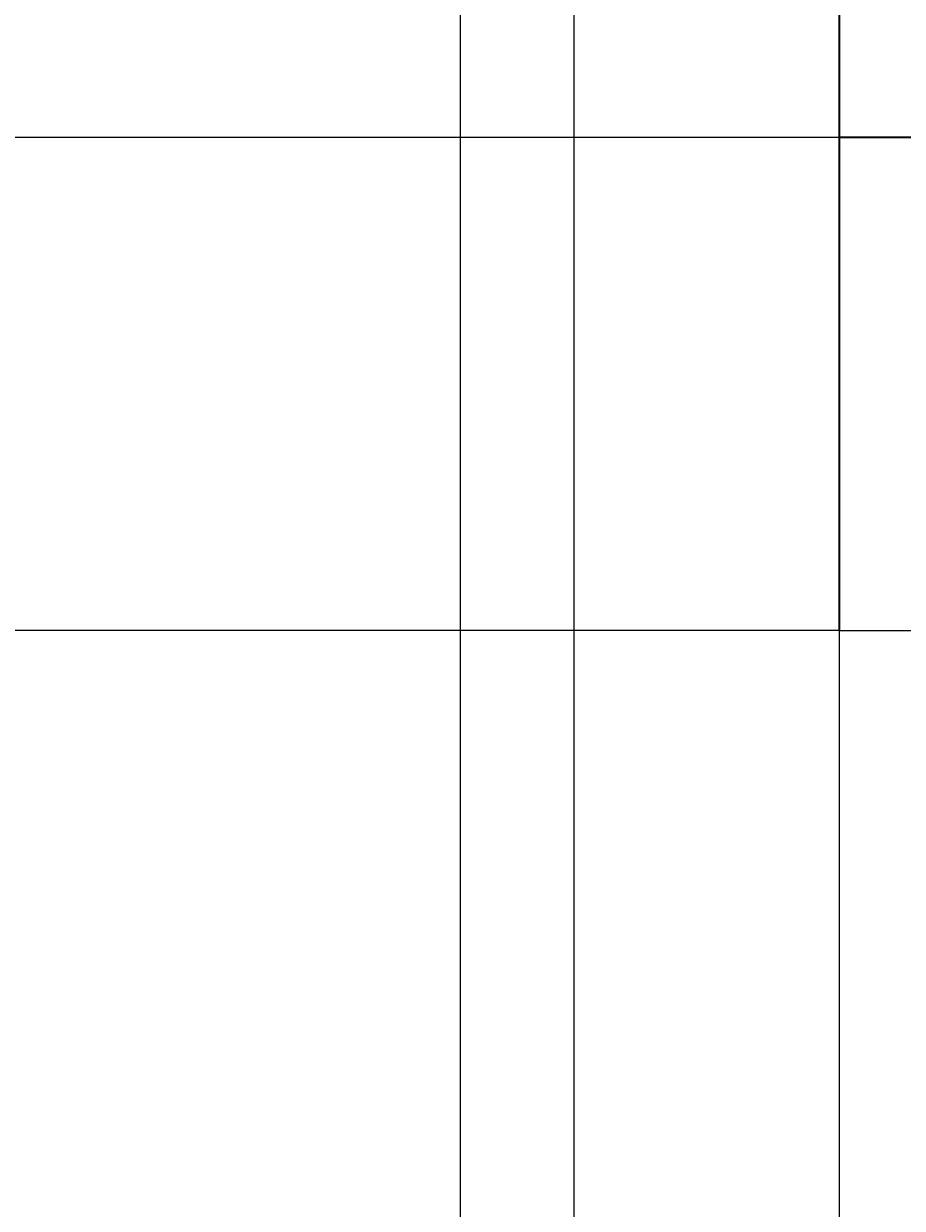
# Model space of a CAD drawing. Units: inches. Extents: x 867 to 1667, y -234 to 788.
# Tile 6 of 42: x 1006 to 1076, y -102 to -8. Entities that reach past the tile are written whole.
import ezdxf

# ---------------------------------------------------------------- set-up
doc = ezdxf.new("R2010")
doc.units = ezdxf.units.IN
doc.header["$MEASUREMENT"] = 0
for name, color, linetype, lineweight in [('A-ANNO-DIMS', 2, 'Continuous', 18), ('A-FLOR-OTLN', 7, 'Continuous', 25), ('A-Wall', 7, 'Continuous', 35)]:
    doc.layers.add(name, color=color, linetype=linetype, lineweight=lineweight)
doc.styles.get("Standard").update_dxf_attribs({"font": 'arial.ttf'})
doc.dimstyles.get("Standard").update_dxf_attribs({"dimtxt": 0.6875, "dimasz": 0.18, "dimexe": 0.18, "dimexo": 0.0625, "dimgap": 0.09, "dimtad": 0, "dimdec": 4, "dimzin": 0, "dimdsep": 46, "dimlunit": 4, "dimtxsty": 'Standard', "dimcen": 0.09, "dimadec": 0, "dimazin": 0, "dimtfac": 1, "dimtdec": 4, "dimtofl": 0, "dimtmove": 0, "dimatfit": 3, "dimfxl": 1, "dimtolj": 1, "dimtzin": 0, "dimarcsym": 0})

# ---------------------------------------------------------------- blocks, each defined once
blk = doc.blocks.new('*D25')
at = {"layer": 'A-ANNO-DIMS', "color": 0, "lineweight": -2, "transparency": 16777216}
for p, q in [((1070.887, -55.971), (1070.887, -233.538)), ((1006.388, -177.471), (1006.388, -233.538)), ((1006.568, -233.358), (1037.65, -233.358)), ((1070.707, -233.358), (1039.625, -233.358))]:
    blk.add_line(p, q, dxfattribs=at)
at = {"layer": 'A-ANNO-DIMS', "color": 0, "transparency": 16777216}
for points in [[(1006.568, -233.328), (1006.568, -233.388), (1006.388, -233.358)], [(1070.707, -233.328), (1070.707, -233.388), (1070.887, -233.358)]]:
    blk.add_solid(points, dxfattribs=at)
at = {"layer": 'Defpoints', "color": 0, "transparency": 16777216}
for p in [(1070.887, -55.908), (1006.388, -177.408), (1070.887, -233.358)]:
    blk.add_point(p, dxfattribs=at)
at = {"layer": 'A-ANNO-DIMS', "color": 0, "transparency": 16777216, "insert": (1038.637, -233.358), "char_height": 0.6875, "attachment_point": 5}
blk.add_mtext('\\A1;64.5', dxfattribs=at)
blk = doc.blocks.new('*D27')
at = {"layer": 'A-ANNO-DIMS', "color": 0, "lineweight": -2, "transparency": 16777216}
for p, q in [((1070.887, -55.971), (1070.887, -233.538)), ((1525.265, -186.471), (1525.265, -233.538)), ((1071.067, -233.358), (1296.813, -233.358)), ((1525.085, -233.358), (1299.338, -233.358))]:
    blk.add_line(p, q, dxfattribs=at)
at = {"layer": 'A-ANNO-DIMS', "color": 0, "transparency": 16777216}
for points in [[(1071.067, -233.328), (1071.067, -233.388), (1070.887, -233.358)], [(1525.085, -233.328), (1525.085, -233.388), (1525.265, -233.358)]]:
    blk.add_solid(points, dxfattribs=at)
at = {"layer": 'Defpoints', "color": 0, "transparency": 16777216}
for p in [(1070.887, -55.908), (1525.265, -186.408), (1525.265, -233.358)]:
    blk.add_point(p, dxfattribs=at)
at = {"layer": 'A-ANNO-DIMS', "color": 0, "transparency": 16777216, "insert": (1298.076, -233.358), "char_height": 0.6875, "attachment_point": 5}
blk.add_mtext('\\A1;454.4', dxfattribs=at)
blk = doc.blocks.new('*D37')
at = {"layer": 'A-ANNO-DIMS', "color": 0, "lineweight": -2, "transparency": 16777216}
for p, q in [((1049.887, 257.555), (1049.887, -233.538)), ((1196.887, 257.555), (1196.887, -233.538)), ((1050.067, -233.358), (1122.569, -233.358)), ((1196.707, -233.358), (1124.204, -233.358))]:
    blk.add_line(p, q, dxfattribs=at)
at = {"layer": 'A-ANNO-DIMS', "color": 0, "transparency": 16777216}
for points in [[(1050.067, -233.328), (1050.067, -233.388), (1049.887, -233.358)], [(1196.707, -233.328), (1196.707, -233.388), (1196.887, -233.358)]]:
    blk.add_solid(points, dxfattribs=at)
at = {"layer": 'Defpoints', "color": 0, "transparency": 16777216}
for p in [(1049.887, 257.617), (1196.887, 257.617), (1196.887, -233.358)]:
    blk.add_point(p, dxfattribs=at)
at = {"layer": 'A-ANNO-DIMS', "color": 0, "transparency": 16777216, "insert": (1123.387, -233.358), "char_height": 0.6875, "attachment_point": 5}
blk.add_mtext('\\A1;147', dxfattribs=at)
blk = doc.blocks.new('*D44')
at = {"layer": 'A-ANNO-DIMS', "color": 0, "lineweight": -2, "transparency": 16777216}
for p, q in [((1070.824, 145.117), (867.757, 145.117)), ((867.937, 144.937), (867.937, 64.931)), ((867.937, -16.703), (867.937, 63.303)), ((1070.824, -16.883), (867.757, -16.883))]:
    blk.add_line(p, q, dxfattribs=at)
at = {"layer": 'A-ANNO-DIMS', "color": 0, "transparency": 16777216}
for points in [[(867.907, 144.937), (867.967, 144.937), (867.937, 145.117)], [(867.907, -16.703), (867.967, -16.703), (867.937, -16.883)]]:
    blk.add_solid(points, dxfattribs=at)
at = {"layer": 'Defpoints', "color": 0, "transparency": 16777216}
for p in [(867.937, 145.117), (1070.887, 145.117), (1070.887, -16.883)]:
    blk.add_point(p, dxfattribs=at)
at = {"layer": 'A-ANNO-DIMS', "color": 0, "transparency": 16777216, "insert": (867.937, 64.117), "char_height": 0.6875, "attachment_point": 5, "rotation": 90}
blk.add_mtext('\\A1;162', dxfattribs=at)
blk = doc.blocks.new('*D47')
at = {"layer": 'A-ANNO-DIMS', "color": 0, "lineweight": -2, "transparency": 16777216}
for p, q in [((1070.824, -16.883), (867.757, -16.883)), ((867.937, -17.063), (867.937, -34.876)), ((867.937, -55.728), (867.937, -37.915)), ((1070.824, -55.908), (867.757, -55.908))]:
    blk.add_line(p, q, dxfattribs=at)
at = {"layer": 'A-ANNO-DIMS', "color": 0, "transparency": 16777216}
for points in [[(867.907, -17.063), (867.967, -17.063), (867.937, -16.883)], [(867.907, -55.728), (867.967, -55.728), (867.937, -55.908)]]:
    blk.add_solid(points, dxfattribs=at)
at = {"layer": 'Defpoints', "color": 0, "transparency": 16777216}
for p in [(867.937, -16.883), (1070.887, -16.883), (1070.887, -55.908)]:
    blk.add_point(p, dxfattribs=at)
at = {"layer": 'A-ANNO-DIMS', "color": 0, "transparency": 16777216, "insert": (867.937, -36.396), "char_height": 0.6875, "attachment_point": 5, "rotation": 90}
blk.add_mtext('\\A1;39.025', dxfattribs=at)
blk = doc.blocks.new('*D49')
at = {"layer": 'A-ANNO-DIMS', "color": 0, "lineweight": -2, "transparency": 16777216}
for p, q in [((1070.887, -55.971), (1070.887, -233.538)), ((1211.887, -55.971), (1211.887, -233.538)), ((1071.067, -233.358), (1140.636, -233.358)), ((1211.707, -233.358), (1142.137, -233.358))]:
    blk.add_line(p, q, dxfattribs=at)
at = {"layer": 'A-ANNO-DIMS', "color": 0, "transparency": 16777216}
for points in [[(1071.067, -233.328), (1071.067, -233.388), (1070.887, -233.358)], [(1211.707, -233.328), (1211.707, -233.388), (1211.887, -233.358)]]:
    blk.add_solid(points, dxfattribs=at)
at = {"layer": 'Defpoints', "color": 0, "transparency": 16777216}
for p in [(1070.887, -55.908), (1211.887, -55.908), (1211.887, -233.358)]:
    blk.add_point(p, dxfattribs=at)
at = {"layer": 'A-ANNO-DIMS', "color": 0, "transparency": 16777216, "insert": (1141.387, -233.358), "char_height": 0.6875, "attachment_point": 5}
blk.add_mtext('\\A1;141', dxfattribs=at)
blk = doc.blocks.new('*D63')
at = {"layer": 'A-ANNO-DIMS', "color": 0, "lineweight": -2, "transparency": 16777216}
for p, q in [((1040.887, 257.555), (1040.887, -233.538)), ((1070.887, 221.555), (1070.887, -233.538)), ((1041.067, -233.358), (1055.306, -233.358)), ((1070.707, -233.358), (1056.468, -233.358))]:
    blk.add_line(p, q, dxfattribs=at)
at = {"layer": 'A-ANNO-DIMS', "color": 0, "transparency": 16777216}
for points in [[(1041.067, -233.328), (1041.067, -233.388), (1040.887, -233.358)], [(1070.707, -233.328), (1070.707, -233.388), (1070.887, -233.358)]]:
    blk.add_solid(points, dxfattribs=at)
at = {"layer": 'Defpoints', "color": 0, "transparency": 16777216}
for p in [(1040.887, 257.617), (1070.887, 221.617), (1070.887, -233.358)]:
    blk.add_point(p, dxfattribs=at)
at = {"layer": 'A-ANNO-DIMS', "color": 0, "transparency": 16777216, "insert": (1055.887, -233.358), "char_height": 0.6875, "attachment_point": 5}
blk.add_mtext('\\A1;30', dxfattribs=at)

msp = doc.modelspace()

# ---------------------------------------------------------------- linework, layer by layer
at = {"layer": 'A-FLOR-OTLN'}
msp.add_line((1070.8866, -55.9081), (1283.8866, -55.9081), dxfattribs=at)
at = {"layer": 'A-Wall'}
for p, q in [((1070.8866, 221.617), (1070.8866, -55.9081)), ((1283.8866, -16.883), (1070.8866, -16.883))]:
    msp.add_line(p, q, dxfattribs=at)

# ---------------------------------------------------------------- dimensions: what is measured, and where the dimension line sits
at = {"layer": 'A-ANNO-DIMS'}
for base, p1, p2, override, picture, middle in [((1070.8866, -233.3581), (1040.8866, 257.617), (1070.8866, 221.617), {"dimdec": 0, "dimlfac": 1, "dimrnd": 0, "dimzin": 0, "dimdsep": 46, "dimlunit": 2}, '*D63', (1055.8866, -233.3581)), ((1196.8866, -233.3581), (1049.8866, 257.617), (1196.8866, 257.617), {"dimdec": 0, "dimlfac": 1, "dimrnd": 0, "dimzin": 0, "dimdsep": 46, "dimlunit": 2}, '*D37', (1123.3866, -233.3581)), ((1070.8866, -233.3581), (1006.3882, -177.4081), (1070.8866, -55.9081), {"dimdec": 1, "dimlfac": 1, "dimrnd": 0, "dimzin": 0, "dimdsep": 46, "dimlunit": 2}, '*D25', (1038.6374, -233.3581)), ((1525.2648, -233.3581), (1070.8866, -55.9081), (1525.2648, -186.4081), {"dimdec": 1, "dimlfac": 1, "dimrnd": 0, "dimzin": 0, "dimdsep": 46, "dimlunit": 2}, '*D27', (1298.0757, -233.3581)), ((1211.8866, -233.3581), (1070.8866, -55.9081), (1211.8866, -55.9081), {"dimdec": 0, "dimlfac": 1, "dimrnd": 0, "dimzin": 0, "dimdsep": 46, "dimlunit": 2}, '*D49', (1141.3866, -233.3581))]:
    dim = msp.add_linear_dim(base=base, p1=p1, p2=p2, dimstyle='Standard', override=override, dxfattribs=at)
    dim.commit()
    dim.dimension.update_dxf_attribs({"geometry": picture, "text_midpoint": middle})
for base, p1, p2, override, picture, middle in [((867.9366, 145.117), (1070.8866, -16.883), (1070.8866, 145.117), {"dimdec": 0, "dimlfac": 1, "dimrnd": 0, "dimzin": 0, "dimdsep": 46, "dimlunit": 2}, '*D44', (867.9366, 64.117)), ((867.9366, -16.883), (1070.8866, -55.9081), (1070.8866, -16.883), {"dimdec": 3, "dimlfac": 1, "dimrnd": 0, "dimzin": 0, "dimdsep": 46, "dimlunit": 2}, '*D47', (867.9366, -36.3955))]:
    dim = msp.add_linear_dim(base=base, p1=p1, p2=p2, angle=90, dimstyle='Standard', override=override, dxfattribs=at)
    dim.commit()
    dim.dimension.update_dxf_attribs({"geometry": picture, "text_midpoint": middle})

doc.saveas('drawing.dxf')
